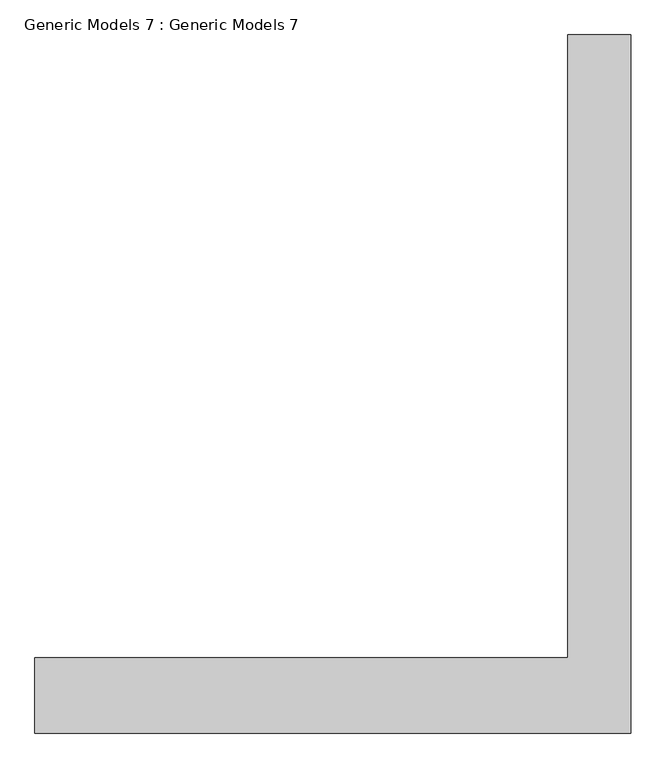
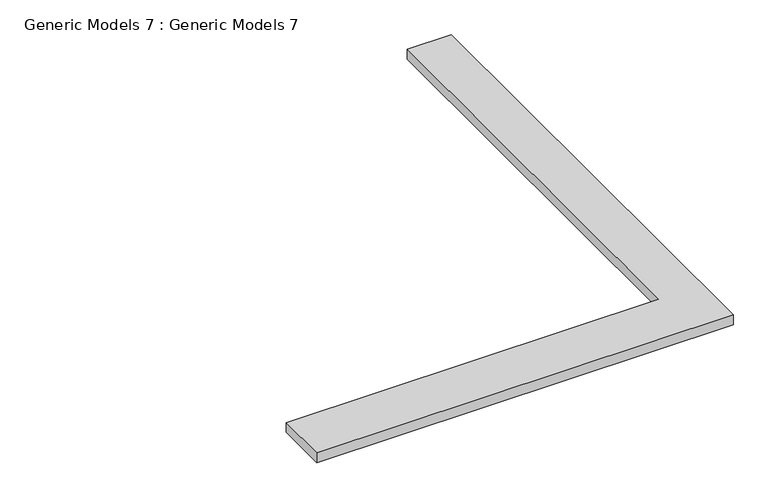
"""IFC4 building model written with IfcOpenShell, lengths in millimetres: proxy geometry, Generic Models 7 : Generic Models 7."""

from ifc_helpers import new_model, si_unit, frame, origin, place, context, project, spatial, polyline, outline, extrude, source, transform, mapped, element, save


def generic_models_7_generic_models_7_15f6dc16(model_context):
    return source(origin(), model_context, "Body", "SweptSolid", [
        extrude(outline(polyline([(-800.7793301, -7462.3015118), (-483.5006493, -7462.3015118), (-483.5006493, -10992.9015118), (-3495.9020237, -10992.9015118), (-3495.9020237, -10611.9015118), (-800.7793301, -10611.9015118), (-800.7793301, -7462.3015118)])), frame((0.0, 0.0, 4135.5328571), z_axis=(0.0, 0.0, 1.0), x_axis=(1.0, 0.0, 0.0)), (0.0, 0.0, 1.0), 76.2),
    ])


if __name__ == "__main__":
    model = new_model("IFC4")
    model_context = context("Model", 3, world=origin())
    ifc_project = project(units=[si_unit("LENGTHUNIT", "METRE", prefix="MILLI")], contexts=[model_context])
    site = spatial("IfcSite", under=ifc_project)
    building = spatial("IfcBuilding", under=site)
    placement = place(None, origin())
    generic_models_7_generic_models_7_shape = generic_models_7_generic_models_7_15f6dc16(model_context)
    element("IfcBuildingElementProxy", 1, Name="Generic Models 7 : Generic Models 7", ObjectType="Generic Models 7 : Generic Models 7", at=placement, inside=building, context=model_context, shape_type="MappedRepresentation", body=[
        mapped(generic_models_7_generic_models_7_shape, transform((0.0, 0.0, 0.0), x_axis=(1.0, 0.0, 0.0), y_axis=(0.0, 1.0, 0.0), z_axis=(0.0, 0.0, 1.0))),
    ])
    save(model, "model.ifc")
